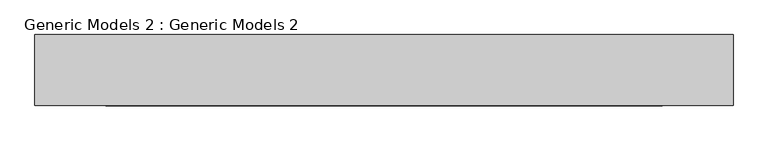
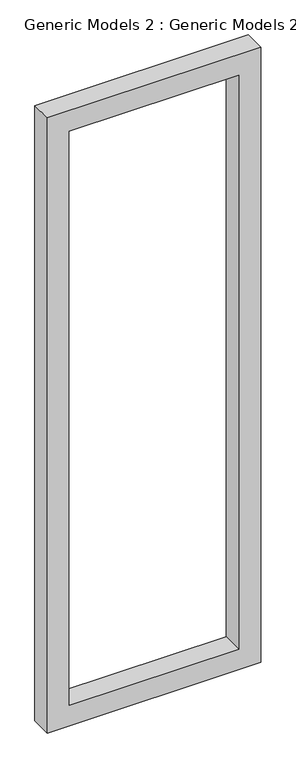
"""IFC4 building model written with IfcOpenShell, lengths in millimetres: proxy geometry, Generic Models 2 : Generic Models 2."""

from ifc_helpers import new_model, si_unit, frame, origin, place, context, project, spatial, polyline, outline, extrude, source, transform, mapped, element, save


def generic_models_2_generic_models_2_798ec4a6(model_context):
    return source(origin(), model_context, "Body", "SweptSolid", [
        extrude(outline(polyline([(12003.5190306, -12351.3456086), (12003.5190306, -13849.9456086), (7431.5190306, -13849.9456086), (7431.5190306, -12351.3456086), (12003.5190306, -12351.3456086)]), holes=[polyline([(11851.1190306, -12503.7456086), (7583.9190306, -12503.7456086), (7583.9190306, -13697.5456086), (11851.1190306, -13697.5456086), (11851.1190306, -12503.7456086)])]), frame((0.0, -11421.2679047, 0.0), z_axis=(0.0, 1.0, 0.0), x_axis=(0.0, 0.0, 1.0)), (0.0, 0.0, 1.0), 152.4),
    ])


if __name__ == "__main__":
    model = new_model("IFC4")
    model_context = context("Model", 3, world=origin())
    ifc_project = project(units=[si_unit("LENGTHUNIT", "METRE", prefix="MILLI")], contexts=[model_context])
    site = spatial("IfcSite", under=ifc_project)
    building = spatial("IfcBuilding", under=site)
    placement = place(None, origin())
    generic_models_2_generic_models_2_shape = generic_models_2_generic_models_2_798ec4a6(model_context)
    element("IfcBuildingElementProxy", 1, Name="Generic Models 2 : Generic Models 2", ObjectType="Generic Models 2 : Generic Models 2", at=placement, inside=building, context=model_context, shape_type="MappedRepresentation", body=[
        mapped(generic_models_2_generic_models_2_shape, transform((0.0, 0.0, 0.0), x_axis=(1.0, 0.0, 0.0), y_axis=(0.0, 1.0, 0.0), z_axis=(0.0, 0.0, 1.0))),
    ])
    save(model, "model.ifc")

# Revit data of these elements
# Element 1 (IfcBuildingElementProxy, "Generic Models 2 : Generic Models 2")
#   Materials on its faces: "WALL ACCENT 6\""
# Materials
#   "WALL ACCENT 6\"": class "Generic", colour RGB 120 120 120, transparency 0, Cost = 0
